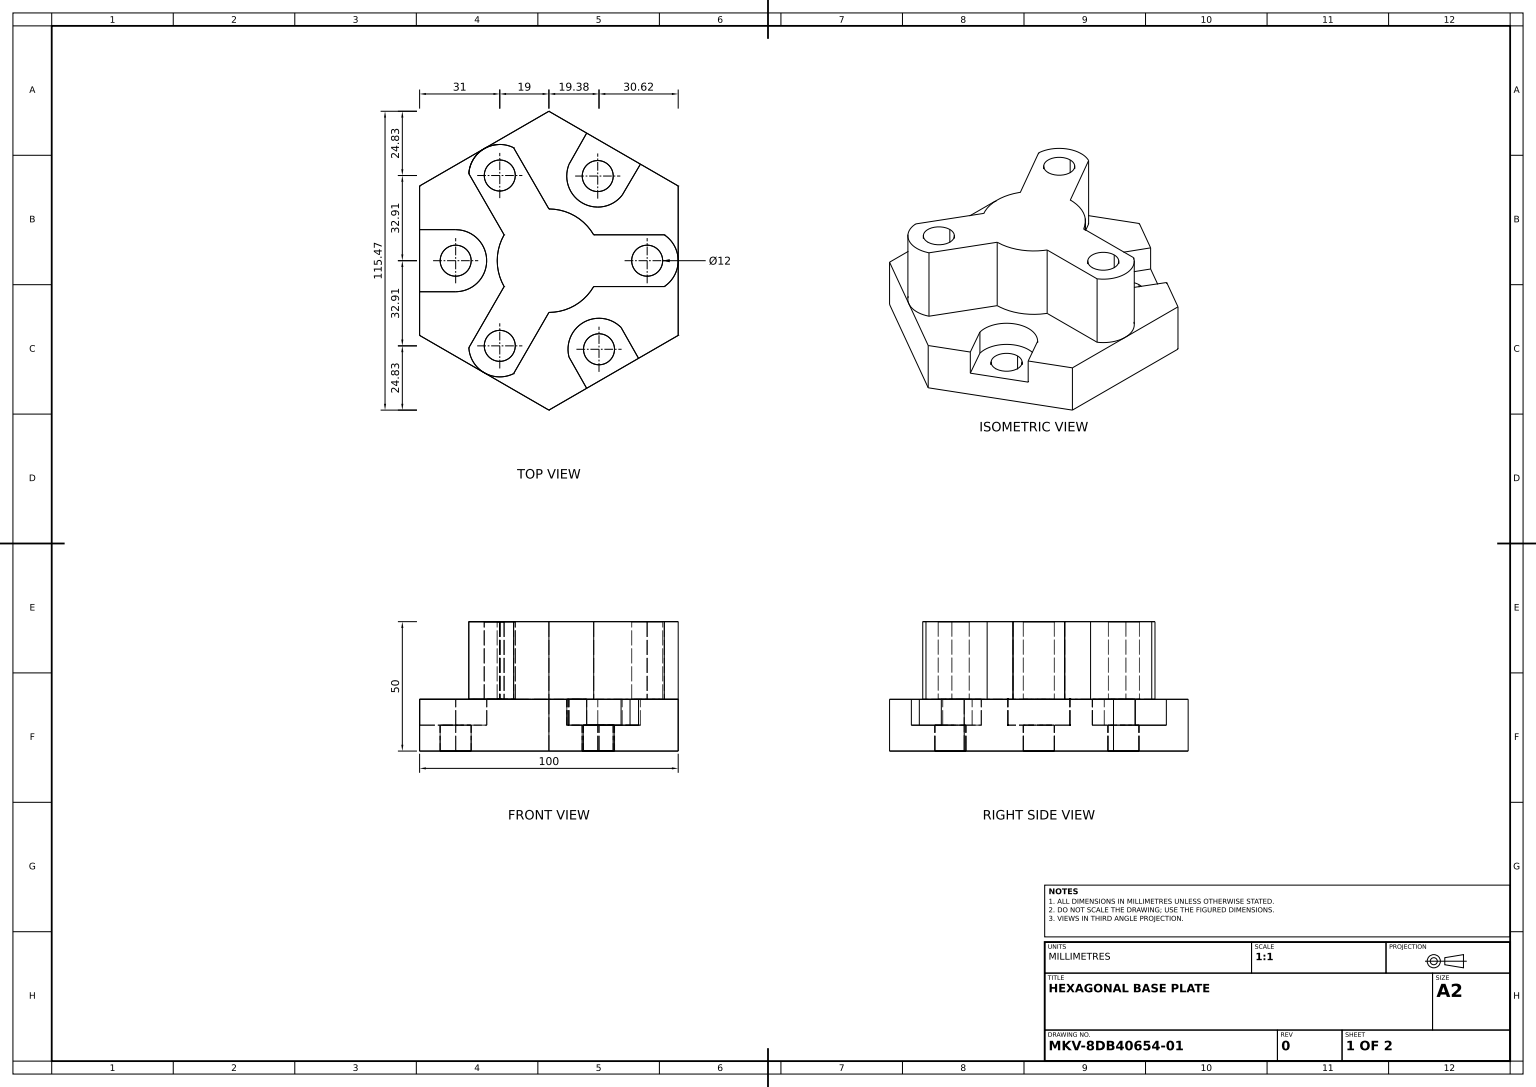
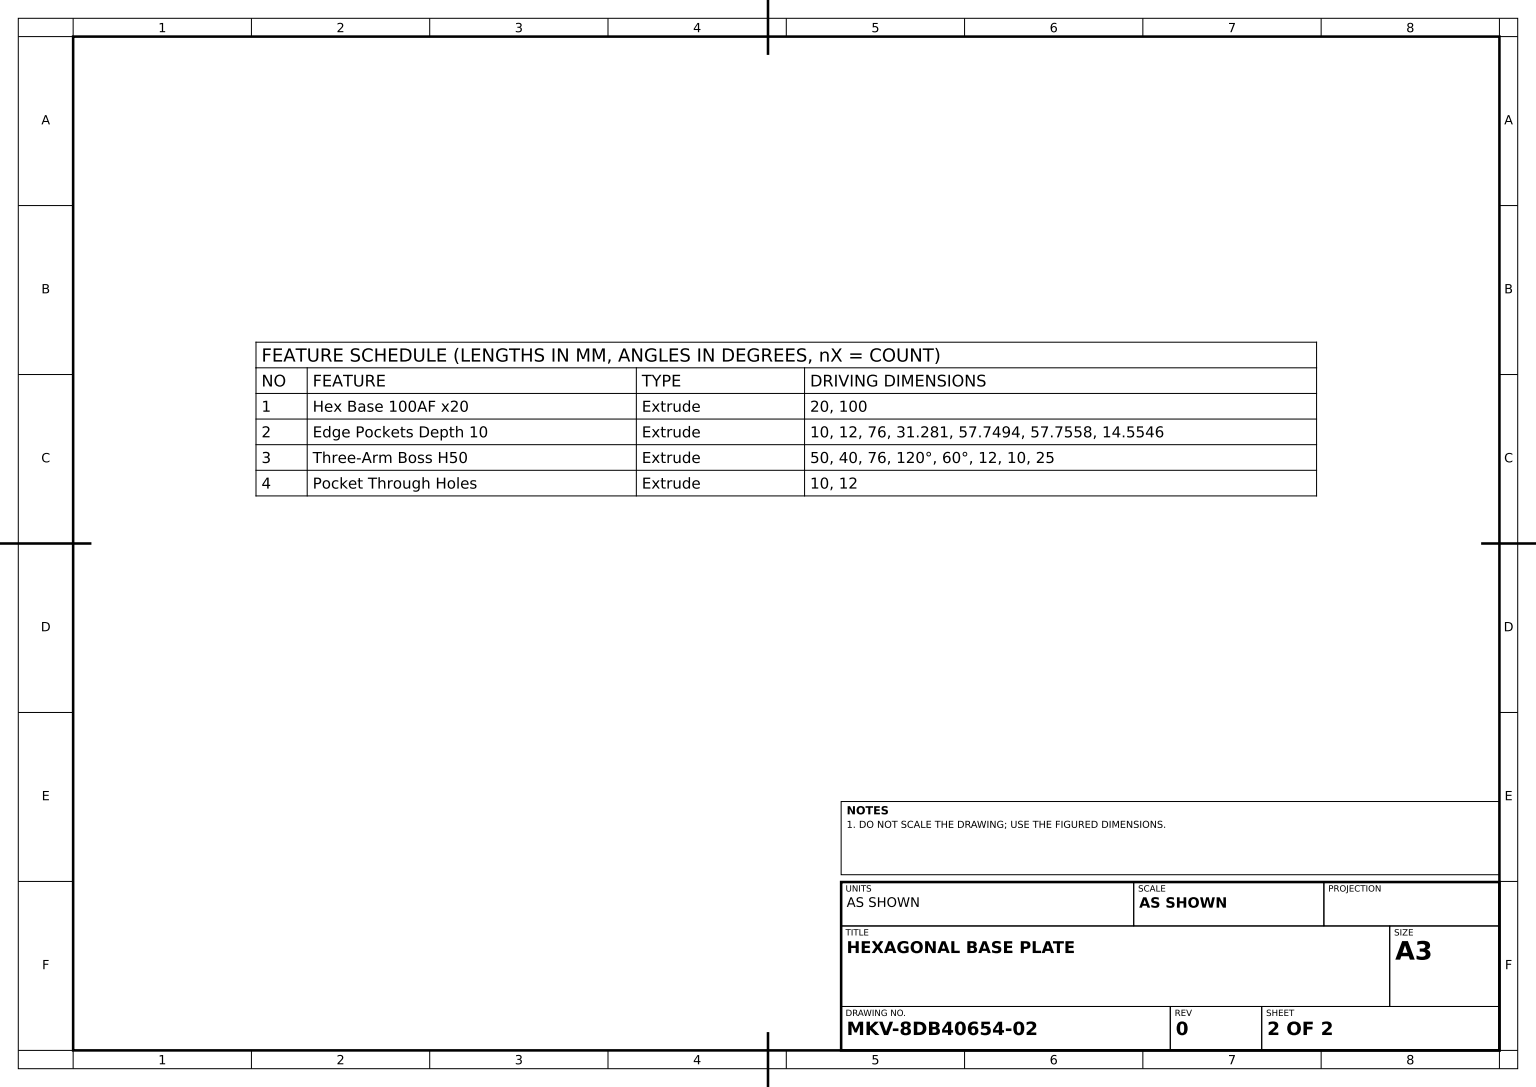
SolidWorks part; units mm, degrees
material "Plain Carbon Steel"
ref_plane "Front Plane" through (0, 0, 0) normal (0, 0, 1) x (1, 0, 0)
ref_plane "Top Plane" through (0, 0, 0) normal (0, 1, 0) x (1, 0, 0)
ref_plane "Right Plane" through (0, 0, 0) normal (1, 0, 0) x (0, 0, -1)
sketch "Hex Base Sketch" plane through (0, 0, 0) normal (0, 1, 0) x (1, 0, 0)
  line L1 (0, 57.735) -> (-50, 28.8675)
  line L2 (-50, 28.8675) -> (-50, -28.8675)
  line L3 (-50, -28.8675) -> (0, -57.735)
  line L4 (0, -57.735) -> (50, -28.8675)
  line L5 (50, -28.8675) -> (50, 28.8675)
  line L6 (50, 28.8675) -> (0, 57.735)
  circle A0 centre (0, 0) radius 50 construction
  dimension "D1" = 100
extrude "Hex Base 100AF x20" add sketch "Hex Base Sketch" along normal blind 20
sketch "Edge Pocket Sketch" plane through (0, 20, 0) normal (0, 1, 0) x (1, 0, 0)
  line L0 (0, 57.735) -> (0, -57.735) construction
  line L1 (-50, 0) -> (50, 0) construction
  line L2 (-50, 28.8675) -> (-50, -28.8675) construction
  line L3 (50, -28.8675) -> (50, 28.8675) construction
  line L4 (0, 0) -> (-24.9303, 43.1805) construction
  line L5 (0, 0) -> (25, 0) construction
  line L6 (0, 0) -> (24.9303, 43.1805) construction
  line L7 (0, 0) -> (-24.6797, -43.6001) construction
  line L8 (0, 0) -> (15.7633, -27.8481)
  line L9 (-50, -12) -> (-50, 12)
  line L10 (-50, 12) -> (-36.0555, 12)
  line L11 (-50, -12) -> (-36.0555, -12)
  line L12 (34.7587, -37.8949) -> (14.6007, -49.3053)
  line L13 (0, -57.735) -> (50, -28.8675) construction
  line L14 (18.719, -33.0696) -> (24.6797, -43.6001) construction
  line L15 (28.7979, -27.3645) -> (34.7587, -37.8949)
  line L16 (8.64, -38.7748) -> (14.6007, -49.3053)
  line L17 (8.64, -38.7748) -> (7.7494, -37.2014)
  line L18 (28.7979, -27.3645) -> (27.9073, -25.7911)
  line L19 (14.6077, 49.3013) -> (35.3923, 37.3013)
  line L20 (50, 28.8675) -> (0, 57.735) construction
  line L21 (14.6077, 49.3013) -> (7.7558, 37.2001)
  line L22 (24.9303, 43.1805) -> (25, 43.3013) construction
  line L23 (35.3923, 37.3013) -> (28.3383, 25.3168)
  circle A0 centre (0, 0) radius 38 construction
  circle A1 centre (19, 32.909) radius 6
  circle A2 centre (38, 0) radius 6
  circle A3 centre (18.719, -33.0696) radius 6
  circle A4 centre (-18.719, -33.0696) radius 6
  circle A5 centre (-38, 0) radius 6
  circle A6 centre (-19, 32.909) radius 6
  arc A7 (-36.0555, 12) -> (-36.0555, -12) centre (-36.0555, 0) cw
  arc A8 (7.7494, -37.2014) -> (27.9073, -25.7911) centre (19.3756, -34.2297) cw
  arc A9 (28.3383, 25.3168) -> (7.7558, 37.2001) centre (18.8817, 32.7041) cw
  dimension "D1" = 12
  dimension "D2" = 12
  dimension "D3" = 12
  dimension "D4" = 12
  dimension "D5" = 76
  dimension "D6" = 31.281
  dimension "D7" = 57.7494
  dimension "D8" = 57.7558
  dimension "D9" = 14.5546
extrude "Edge Pockets Depth 10" cut sketch "Edge Pocket Sketch" against normal blind 10
sketch "Three-Arm Boss Sketch" plane through (0, 0, 0) normal (0, 1, 0) x (1, 0, 0)
  line L0 (0, 0) -> (-25, -43.3013) construction
  line L1 (0, 0) -> (-25, 43.3013) construction
  line L2 (-50, -28.8675) -> (0, -57.735) construction
  line L3 (0, 0) -> (50, 0) construction
  line L4 (0, 57.735) -> (-50, 28.8675) construction
  line L5 (50, -28.8675) -> (50, 28.8675) construction
  line L6 (17.3205, -10) -> (44.6332, -10)
  line L8 (-17.3205, -10) -> (-30.9769, -33.6535)
  line L9 (0, 20) -> (-13.6564, 43.6535)
  line L10 (17.3205, 10) -> (44.6332, 10)
  line L11 (0, -20) -> (-13.6564, -43.6535)
  line L12 (-17.3205, 10) -> (-30.9769, 33.6535)
  line L13 (-8.6603, 5) -> (-33.6603, -38.3013) construction
  line L14 (8.6603, -5) -> (-16.3397, -48.3013) construction
  line L15 (0, 10) -> (50, 10) construction
  line L17 (25, -10) -> (25, 10)
  circle A0 centre (0, 0) radius 38 construction
  circle A1 centre (-38, 0) radius 6
  circle A2 centre (-19, -32.909) radius 6
  circle A3 centre (38, 0) radius 6
  circle A4 centre (-19, 32.909) radius 6
  arc A5 (0, -20) -> (17.3205, -10) centre (0, 0) ccw
  arc A6 (-17.3205, 10) -> (-17.3205, -10) centre (0, 0) ccw
  arc A7 (17.3205, 10) -> (0, 20) centre (0, 0) ccw
  arc A8 (44.6332, -10) -> (44.6332, 10) centre (38, 0) ccw
  arc A10 (-30.9769, -33.6535) -> (-13.6564, -43.6535) centre (-19, -32.909) ccw
  arc A11 (-13.6564, 43.6535) -> (-30.9769, 33.6535) centre (-19, 32.909) ccw
  point P21 (8.6603, 5)
  point P22 (-16.3397, 48.3013)
  point P23 (0, -10)
  point P24 (50, -10)
  point P27 (-8.6603, -5)
  point P28 (-33.6603, 38.3013)
  dimension "D1" = 40
  dimension "D4" = 60
  dimension "D2" = 76
  dimension "D5" = 12
  dimension "D6" = 12
  dimension "D3" = 120
  dimension "D7" = 10
  dimension "D8" = 10
  dimension "D9" = 10
  dimension "D10" = 10
  dimension "D11" = 10
  dimension "D12" = 25
extrude "Three-Arm Boss H50" add sketch "Three-Arm Boss Sketch" along normal blind 50 contours L9 A11 L12 A6 L8 A10 L11 A5 L6 L17 L10 A7 A2 A4 | L6 A8 L10 L17 A3
sketch "Pocket Hole Sketch" plane through (0, 10, 0) normal (0, 1, 0) x (1, 0, 0)
  circle A0 centre (19.3756, -34.2297) radius 6
  circle A1 centre (-36.0555, 0) radius 6
  circle A2 centre (18.8817, 32.7041) radius 6
  dimension "D1" = 12
extrude "Pocket Through Holes" cut sketch "Pocket Hole Sketch" against normal blind 10
